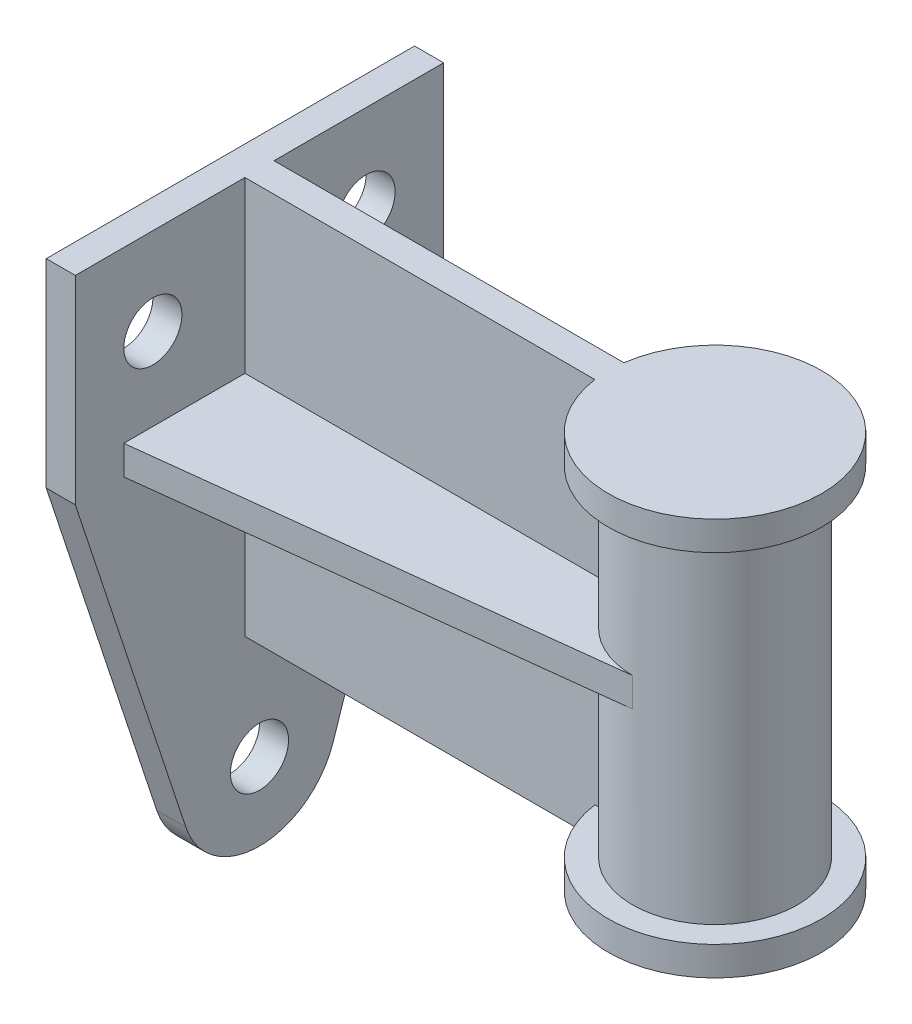
ISO-10303-21;
HEADER;
FILE_DESCRIPTION(('STEP AP214'),'2;1');
FILE_NAME('part.step','',(''),(''),'','','');
FILE_SCHEMA(('AUTOMOTIVE_DESIGN { 1 0 10303 214 1 1 1 1 }'));
ENDSEC;
DATA;
#1=APPLICATION_CONTEXT('core data for automotive mechanical design processes');
#2=APPLICATION_PROTOCOL_DEFINITION('international standard','automotive_design',2000,#1);
#3=PRODUCT_CONTEXT('',#1,'mechanical');
#4=PRODUCT('Part','Part','',(#3));
#5=PRODUCT_RELATED_PRODUCT_CATEGORY('part','',(#4));
#6=PRODUCT_DEFINITION_FORMATION('','',#4);
#7=PRODUCT_DEFINITION_CONTEXT('part definition',#1,'design');
#8=PRODUCT_DEFINITION('design','',#6,#7);
#9=PRODUCT_DEFINITION_SHAPE('','',#8);
#10=(LENGTH_UNIT() NAMED_UNIT(*) SI_UNIT(.MILLI.,.METRE.));
#11=(NAMED_UNIT(*) PLANE_ANGLE_UNIT() SI_UNIT($,.RADIAN.));
#12=(NAMED_UNIT(*) SI_UNIT($,.STERADIAN.) SOLID_ANGLE_UNIT());
#13=UNCERTAINTY_MEASURE_WITH_UNIT(LENGTH_MEASURE(1.E-05),#10,'distance_accuracy_value','');
#14=(GEOMETRIC_REPRESENTATION_CONTEXT(3) GLOBAL_UNCERTAINTY_ASSIGNED_CONTEXT((#13)) GLOBAL_UNIT_ASSIGNED_CONTEXT((#10,
#11,#12)) REPRESENTATION_CONTEXT('',''));
#15=CARTESIAN_POINT('',(0.,0.,0.));
#16=DIRECTION('',(0.,0.,1.));
#17=DIRECTION('',(1.,0.,0.));
#18=AXIS2_PLACEMENT_3D('',#15,#16,#17);
#19=CARTESIAN_POINT('',(0.,41.,0.));
#20=DIRECTION('',(0.,1.,0.));
#21=DIRECTION('',(0.,0.,1.));
#22=AXIS2_PLACEMENT_3D('',#19,#20,#21);
#23=PLANE('',#22);
#24=CARTESIAN_POINT('',(0.,41.,0.));
#25=DIRECTION('',(0.,1.,0.));
#26=DIRECTION('',(0.,0.,1.));
#27=AXIS2_PLACEMENT_3D('',#24,#25,#26);
#28=CIRCLE('',#27,17.);
#29=CARTESIAN_POINT('',(-7.7142620860374,41.,-15.148932651112));
#30=VERTEX_POINT('',#29);
#31=CARTESIAN_POINT('',(-16.7332005306815,41.,-3.));
#32=VERTEX_POINT('',#31);
#33=EDGE_CURVE('E61',#30,#32,#28,.T.);
#34=ORIENTED_EDGE('',*,*,#33,.T.);
#35=DIRECTION('',(1.,0.,0.));
#36=VECTOR('',#35,1.);
#37=CARTESIAN_POINT('',(0.,41.,-3.));
#38=LINE('',#37,#36);
#39=CARTESIAN_POINT('',(-94.,41.,-3.));
#40=VERTEX_POINT('',#39);
#41=EDGE_CURVE('E197',#40,#32,#38,.T.);
#42=ORIENTED_EDGE('',*,*,#41,.F.);
#43=DIRECTION('',(0.,0.,1.));
#44=VECTOR('',#43,1.);
#45=CARTESIAN_POINT('',(-94.,41.,0.));
#46=LINE('',#45,#44);
#47=CARTESIAN_POINT('',(-94.,41.,-28.));
#48=VERTEX_POINT('',#47);
#49=EDGE_CURVE('E11',#48,#40,#46,.T.);
#50=ORIENTED_EDGE('',*,*,#49,.F.);
#51=DIRECTION('',(0.989090177881817,0.,0.147311303088781));
#52=VECTOR('',#51,1.);
#53=CARTESIAN_POINT('',(2.03985828166519,41.,-13.696191319752));
#54=LINE('',#53,#52);
#55=EDGE_CURVE('E310',#48,#30,#54,.T.);
#56=ORIENTED_EDGE('',*,*,#55,.T.);
#57=EDGE_LOOP('',(#34,#42,#50,#56));
#58=FACE_BOUND('',#57,.T.);
#59=ADVANCED_FACE('F41',(#58),#23,.F.);
#60=CARTESIAN_POINT('',(-94.,41.,3.));
#61=VERTEX_POINT('',#60);
#62=CARTESIAN_POINT('',(-94.,41.,28.));
#63=VERTEX_POINT('',#62);
#64=EDGE_CURVE('E47',#61,#63,#46,.T.);
#65=ORIENTED_EDGE('',*,*,#64,.F.);
#66=DIRECTION('',(-1.,0.,0.));
#67=VECTOR('',#66,1.);
#68=CARTESIAN_POINT('',(0.,41.,3.));
#69=LINE('',#68,#67);
#70=CARTESIAN_POINT('',(-16.7332005306815,41.,3.));
#71=VERTEX_POINT('',#70);
#72=EDGE_CURVE('E186',#71,#61,#69,.T.);
#73=ORIENTED_EDGE('',*,*,#72,.F.);
#74=CARTESIAN_POINT('',(0.,41.,17.));
#75=VERTEX_POINT('',#74);
#76=EDGE_CURVE('E214',#71,#75,#28,.T.);
#77=ORIENTED_EDGE('',*,*,#76,.T.);
#78=DIRECTION('',(0.99322253932129,0.,-0.116228169495045));
#79=VECTOR('',#78,1.);
#80=CARTESIAN_POINT('',(1.96248743999107,41.,16.7703472144691));
#81=LINE('',#80,#79);
#82=EDGE_CURVE('E215',#63,#75,#81,.T.);
#83=ORIENTED_EDGE('',*,*,#82,.F.);
#84=EDGE_LOOP('',(#65,#73,#77,#83));
#85=FACE_BOUND('',#84,.T.);
#86=ADVANCED_FACE('F208',(#85),#23,.F.);
#87=CARTESIAN_POINT('',(0.,82.,0.));
#88=DIRECTION('',(0.,-1.,0.));
#89=DIRECTION('',(0.,0.,-1.));
#90=AXIS2_PLACEMENT_3D('',#87,#88,#89);
#91=CYLINDRICAL_SURFACE('',#90,17.);
#92=CARTESIAN_POINT('',(0.,6.,0.));
#93=DIRECTION('',(0.,1.,0.));
#94=DIRECTION('',(0.,0.,1.));
#95=AXIS2_PLACEMENT_3D('',#92,#93,#94);
#96=CIRCLE('',#95,17.);
#97=CARTESIAN_POINT('',(-16.7332005306815,6.,3.));
#98=VERTEX_POINT('',#97);
#99=CARTESIAN_POINT('',(-16.7332005306815,6.,-3.));
#100=VERTEX_POINT('',#99);
#101=EDGE_CURVE('E221',#98,#100,#96,.T.);
#102=ORIENTED_EDGE('',*,*,#101,.T.);
#103=DIRECTION('',(0.,-1.,0.));
#104=VECTOR('',#103,1.);
#105=CARTESIAN_POINT('',(-16.7332005306815,82.,-3.));
#106=LINE('',#105,#104);
#107=EDGE_CURVE('E354',#100,#32,#106,.F.);
#108=ORIENTED_EDGE('',*,*,#107,.T.);
#109=ORIENTED_EDGE('',*,*,#33,.F.);
#110=DIRECTION('',(0.,1.,0.));
#111=VECTOR('',#110,1.);
#112=CARTESIAN_POINT('',(-7.71426208603739,41.,-15.148932651112));
#113=LINE('',#112,#111);
#114=CARTESIAN_POINT('',(-7.71426208603739,47.,-15.148932651112));
#115=VERTEX_POINT('',#114);
#116=EDGE_CURVE('E304',#30,#115,#113,.T.);
#117=ORIENTED_EDGE('',*,*,#116,.T.);
#118=CARTESIAN_POINT('',(0.,47.,0.));
#119=DIRECTION('',(0.,1.,0.));
#120=DIRECTION('',(0.,0.,1.));
#121=AXIS2_PLACEMENT_3D('',#118,#119,#120);
#122=CIRCLE('',#121,17.);
#123=CARTESIAN_POINT('',(-16.7332005306815,47.,-3.));
#124=VERTEX_POINT('',#123);
#125=EDGE_CURVE('E319',#115,#124,#122,.T.);
#126=ORIENTED_EDGE('',*,*,#125,.T.);
#127=DIRECTION('',(0.,-1.,0.));
#128=VECTOR('',#127,1.);
#129=CARTESIAN_POINT('',(-16.7332005306815,82.,-3.));
#130=LINE('',#129,#128);
#131=CARTESIAN_POINT('',(-16.7332005306815,76.,-3.));
#132=VERTEX_POINT('',#131);
#133=EDGE_CURVE('E231',#124,#132,#130,.F.);
#134=ORIENTED_EDGE('',*,*,#133,.T.);
#135=CARTESIAN_POINT('',(0.,76.,0.));
#136=DIRECTION('',(0.,1.,0.));
#137=DIRECTION('',(0.,0.,1.));
#138=AXIS2_PLACEMENT_3D('',#135,#136,#137);
#139=CIRCLE('',#138,17.);
#140=CARTESIAN_POINT('',(-16.7332005306815,76.,3.));
#141=VERTEX_POINT('',#140);
#142=EDGE_CURVE('E217',#141,#132,#139,.T.);
#143=ORIENTED_EDGE('',*,*,#142,.F.);
#144=DIRECTION('',(0.,-1.,0.));
#145=VECTOR('',#144,1.);
#146=CARTESIAN_POINT('',(-16.7332005306815,82.,3.));
#147=LINE('',#146,#145);
#148=CARTESIAN_POINT('',(-16.7332005306815,47.,3.));
#149=VERTEX_POINT('',#148);
#150=EDGE_CURVE('E245',#149,#141,#147,.F.);
#151=ORIENTED_EDGE('',*,*,#150,.F.);
#152=CARTESIAN_POINT('',(0.,47.,0.));
#153=DIRECTION('',(0.,1.,0.));
#154=DIRECTION('',(0.,0.,1.));
#155=AXIS2_PLACEMENT_3D('',#152,#153,#154);
#156=CIRCLE('',#155,17.);
#157=CARTESIAN_POINT('',(0.,47.,17.));
#158=VERTEX_POINT('',#157);
#159=EDGE_CURVE('E297',#149,#158,#156,.T.);
#160=ORIENTED_EDGE('',*,*,#159,.T.);
#161=DIRECTION('',(0.,1.,0.));
#162=VECTOR('',#161,1.);
#163=CARTESIAN_POINT('',(0.,41.,17.));
#164=LINE('',#163,#162);
#165=EDGE_CURVE('E281',#75,#158,#164,.T.);
#166=ORIENTED_EDGE('',*,*,#165,.F.);
#167=ORIENTED_EDGE('',*,*,#76,.F.);
#168=DIRECTION('',(0.,-1.,0.));
#169=VECTOR('',#168,1.);
#170=CARTESIAN_POINT('',(-16.7332005306815,82.,3.));
#171=LINE('',#170,#169);
#172=EDGE_CURVE('E195',#71,#98,#171,.T.);
#173=ORIENTED_EDGE('',*,*,#172,.T.);
#174=EDGE_LOOP('',(#102,#108,#109,#117,#126,#134,#143,#151,#160,#166,#167,#173));
#175=FACE_BOUND('',#174,.T.);
#176=ADVANCED_FACE('F43',(#175),#91,.T.);
#177=CARTESIAN_POINT('',(0.,6.,0.));
#178=DIRECTION('',(0.,-1.,0.));
#179=DIRECTION('',(0.,0.,-1.));
#180=AXIS2_PLACEMENT_3D('',#177,#178,#179);
#181=CYLINDRICAL_SURFACE('',#180,22.);
#182=CARTESIAN_POINT('',(0.,0.,0.));
#183=DIRECTION('',(0.,1.,0.));
#184=DIRECTION('',(0.,0.,1.));
#185=AXIS2_PLACEMENT_3D('',#182,#183,#184);
#186=CIRCLE('',#185,22.);
#187=CARTESIAN_POINT('',(-21.7944947177034,0.,3.));
#188=VERTEX_POINT('',#187);
#189=CARTESIAN_POINT('',(-21.7944947177034,0.,-3.));
#190=VERTEX_POINT('',#189);
#191=EDGE_CURVE('E222',#188,#190,#186,.T.);
#192=ORIENTED_EDGE('',*,*,#191,.T.);
#193=DIRECTION('',(0.,-1.,0.));
#194=VECTOR('',#193,1.);
#195=CARTESIAN_POINT('',(-21.7944947177034,6.,-3.));
#196=LINE('',#195,#194);
#197=CARTESIAN_POINT('',(-21.7944947177034,6.,-3.));
#198=VERTEX_POINT('',#197);
#199=EDGE_CURVE('E365',#190,#198,#196,.F.);
#200=ORIENTED_EDGE('',*,*,#199,.T.);
#201=CARTESIAN_POINT('',(0.,6.,0.));
#202=DIRECTION('',(0.,1.,0.));
#203=DIRECTION('',(0.,0.,1.));
#204=AXIS2_PLACEMENT_3D('',#201,#202,#203);
#205=CIRCLE('',#204,22.);
#206=CARTESIAN_POINT('',(-21.7944947177034,6.,3.));
#207=VERTEX_POINT('',#206);
#208=EDGE_CURVE('E216',#207,#198,#205,.T.);
#209=ORIENTED_EDGE('',*,*,#208,.F.);
#210=DIRECTION('',(0.,-1.,0.));
#211=VECTOR('',#210,1.);
#212=CARTESIAN_POINT('',(-21.7944947177034,6.,3.));
#213=LINE('',#212,#211);
#214=EDGE_CURVE('E368',#207,#188,#213,.T.);
#215=ORIENTED_EDGE('',*,*,#214,.T.);
#216=EDGE_LOOP('',(#192,#200,#209,#215));
#217=FACE_BOUND('',#216,.T.);
#218=ADVANCED_FACE('F386',(#217),#181,.T.);
#219=CARTESIAN_POINT('',(0.,6.,0.));
#220=DIRECTION('',(0.,1.,0.));
#221=DIRECTION('',(0.,0.,1.));
#222=AXIS2_PLACEMENT_3D('',#219,#220,#221);
#223=PLANE('',#222);
#224=DIRECTION('',(-1.,0.,0.));
#225=VECTOR('',#224,1.);
#226=CARTESIAN_POINT('',(0.,6.,-3.));
#227=LINE('',#226,#225);
#228=EDGE_CURVE('E362',#100,#198,#227,.T.);
#229=ORIENTED_EDGE('',*,*,#228,.F.);
#230=ORIENTED_EDGE('',*,*,#101,.F.);
#231=DIRECTION('',(1.,0.,0.));
#232=VECTOR('',#231,1.);
#233=CARTESIAN_POINT('',(0.,6.,3.));
#234=LINE('',#233,#232);
#235=EDGE_CURVE('E371',#207,#98,#234,.T.);
#236=ORIENTED_EDGE('',*,*,#235,.F.);
#237=ORIENTED_EDGE('',*,*,#208,.T.);
#238=EDGE_LOOP('',(#229,#230,#236,#237));
#239=FACE_BOUND('',#238,.T.);
#240=ADVANCED_FACE('F387',(#239),#223,.T.);
#241=CARTESIAN_POINT('',(0.,0.,0.));
#242=DIRECTION('',(0.,1.,0.));
#243=DIRECTION('',(0.,0.,1.));
#244=AXIS2_PLACEMENT_3D('',#241,#242,#243);
#245=PLANE('',#244);
#246=ORIENTED_EDGE('',*,*,#191,.F.);
#247=DIRECTION('',(-1.,0.,0.));
#248=VECTOR('',#247,1.);
#249=CARTESIAN_POINT('',(0.,0.,3.));
#250=LINE('',#249,#248);
#251=CARTESIAN_POINT('',(-94.,0.,3.));
#252=VERTEX_POINT('',#251);
#253=EDGE_CURVE('E380',#188,#252,#250,.T.);
#254=ORIENTED_EDGE('',*,*,#253,.T.);
#255=DIRECTION('',(0.,0.,-1.));
#256=VECTOR('',#255,1.);
#257=CARTESIAN_POINT('',(-94.,0.,3.));
#258=LINE('',#257,#256);
#259=CARTESIAN_POINT('',(-94.,0.,-3.));
#260=VERTEX_POINT('',#259);
#261=EDGE_CURVE('E207',#252,#260,#258,.T.);
#262=ORIENTED_EDGE('',*,*,#261,.T.);
#263=DIRECTION('',(1.,0.,0.));
#264=VECTOR('',#263,1.);
#265=CARTESIAN_POINT('',(0.,0.,-3.));
#266=LINE('',#265,#264);
#267=EDGE_CURVE('E200',#260,#190,#266,.T.);
#268=ORIENTED_EDGE('',*,*,#267,.T.);
#269=EDGE_LOOP('',(#246,#254,#262,#268));
#270=FACE_BOUND('',#269,.T.);
#271=ADVANCED_FACE('F395',(#270),#245,.F.);
#272=CARTESIAN_POINT('',(0.,76.,0.));
#273=DIRECTION('',(0.,1.,0.));
#274=DIRECTION('',(0.,0.,1.));
#275=AXIS2_PLACEMENT_3D('',#272,#273,#274);
#276=CYLINDRICAL_SURFACE('',#275,22.);
#277=DIRECTION('',(0.,1.,0.));
#278=VECTOR('',#277,1.);
#279=CARTESIAN_POINT('',(-21.7944947177034,76.,-3.));
#280=LINE('',#279,#278);
#281=CARTESIAN_POINT('',(-21.7944947177034,82.,-3.));
#282=VERTEX_POINT('',#281);
#283=CARTESIAN_POINT('',(-21.7944947177034,76.,-3.));
#284=VERTEX_POINT('',#283);
#285=EDGE_CURVE('E240',#282,#284,#280,.F.);
#286=ORIENTED_EDGE('',*,*,#285,.F.);
#287=CARTESIAN_POINT('',(0.,82.,0.));
#288=DIRECTION('',(0.,1.,0.));
#289=DIRECTION('',(0.,0.,1.));
#290=AXIS2_PLACEMENT_3D('',#287,#288,#289);
#291=CIRCLE('',#290,22.);
#292=CARTESIAN_POINT('',(-21.7944947177034,82.,3.));
#293=VERTEX_POINT('',#292);
#294=EDGE_CURVE('E229',#293,#282,#291,.T.);
#295=ORIENTED_EDGE('',*,*,#294,.F.);
#296=DIRECTION('',(0.,1.,0.));
#297=VECTOR('',#296,1.);
#298=CARTESIAN_POINT('',(-21.7944947177034,76.,3.));
#299=LINE('',#298,#297);
#300=CARTESIAN_POINT('',(-21.7944947177034,76.,3.));
#301=VERTEX_POINT('',#300);
#302=EDGE_CURVE('E242',#293,#301,#299,.F.);
#303=ORIENTED_EDGE('',*,*,#302,.T.);
#304=CARTESIAN_POINT('',(0.,76.,0.));
#305=DIRECTION('',(0.,1.,0.));
#306=DIRECTION('',(0.,0.,1.));
#307=AXIS2_PLACEMENT_3D('',#304,#305,#306);
#308=CIRCLE('',#307,22.);
#309=EDGE_CURVE('E223',#301,#284,#308,.T.);
#310=ORIENTED_EDGE('',*,*,#309,.T.);
#311=EDGE_LOOP('',(#286,#295,#303,#310));
#312=FACE_BOUND('',#311,.T.);
#313=ADVANCED_FACE('F420',(#312),#276,.T.);
#314=CARTESIAN_POINT('',(0.,76.,0.));
#315=DIRECTION('',(0.,1.,0.));
#316=DIRECTION('',(0.,0.,1.));
#317=AXIS2_PLACEMENT_3D('',#314,#315,#316);
#318=PLANE('',#317);
#319=ORIENTED_EDGE('',*,*,#142,.T.);
#320=DIRECTION('',(-1.,0.,0.));
#321=VECTOR('',#320,1.);
#322=CARTESIAN_POINT('',(0.,76.,-3.));
#323=LINE('',#322,#321);
#324=EDGE_CURVE('E239',#132,#284,#323,.T.);
#325=ORIENTED_EDGE('',*,*,#324,.T.);
#326=ORIENTED_EDGE('',*,*,#309,.F.);
#327=DIRECTION('',(-1.,0.,0.));
#328=VECTOR('',#327,1.);
#329=CARTESIAN_POINT('',(0.,76.,3.));
#330=LINE('',#329,#328);
#331=EDGE_CURVE('E250',#141,#301,#330,.T.);
#332=ORIENTED_EDGE('',*,*,#331,.F.);
#333=EDGE_LOOP('',(#319,#325,#326,#332));
#334=FACE_BOUND('',#333,.T.);
#335=ADVANCED_FACE('F424',(#334),#318,.F.);
#336=CARTESIAN_POINT('',(0.,82.,0.));
#337=DIRECTION('',(0.,1.,0.));
#338=DIRECTION('',(0.,0.,1.));
#339=AXIS2_PLACEMENT_3D('',#336,#337,#338);
#340=PLANE('',#339);
#341=ORIENTED_EDGE('',*,*,#294,.T.);
#342=DIRECTION('',(-1.,0.,0.));
#343=VECTOR('',#342,1.);
#344=CARTESIAN_POINT('',(0.,82.,-3.));
#345=LINE('',#344,#343);
#346=CARTESIAN_POINT('',(-94.,82.,-3.));
#347=VERTEX_POINT('',#346);
#348=EDGE_CURVE('E285',#282,#347,#345,.T.);
#349=ORIENTED_EDGE('',*,*,#348,.T.);
#350=DIRECTION('',(0.,0.,-1.));
#351=VECTOR('',#350,1.);
#352=CARTESIAN_POINT('',(-94.,82.,0.));
#353=LINE('',#352,#351);
#354=CARTESIAN_POINT('',(-94.,82.,-38.));
#355=VERTEX_POINT('',#354);
#356=EDGE_CURVE('E276',#347,#355,#353,.T.);
#357=ORIENTED_EDGE('',*,*,#356,.T.);
#358=DIRECTION('',(1.,0.,0.));
#359=VECTOR('',#358,1.);
#360=CARTESIAN_POINT('',(0.,82.,-38.));
#361=LINE('',#360,#359);
#362=CARTESIAN_POINT('',(-100.,82.,-38.));
#363=VERTEX_POINT('',#362);
#364=EDGE_CURVE('E277',#363,#355,#361,.T.);
#365=ORIENTED_EDGE('',*,*,#364,.F.);
#366=DIRECTION('',(0.,0.,-1.));
#367=VECTOR('',#366,1.);
#368=CARTESIAN_POINT('',(-100.,82.,0.));
#369=LINE('',#368,#367);
#370=CARTESIAN_POINT('',(-100.,82.,38.));
#371=VERTEX_POINT('',#370);
#372=EDGE_CURVE('E274',#371,#363,#369,.T.);
#373=ORIENTED_EDGE('',*,*,#372,.F.);
#374=DIRECTION('',(1.,0.,0.));
#375=VECTOR('',#374,1.);
#376=CARTESIAN_POINT('',(0.,82.,38.));
#377=LINE('',#376,#375);
#378=CARTESIAN_POINT('',(-94.,82.,38.));
#379=VERTEX_POINT('',#378);
#380=EDGE_CURVE('E272',#371,#379,#377,.T.);
#381=ORIENTED_EDGE('',*,*,#380,.T.);
#382=DIRECTION('',(0.,0.,-1.));
#383=VECTOR('',#382,1.);
#384=CARTESIAN_POINT('',(-94.,82.,0.));
#385=LINE('',#384,#383);
#386=CARTESIAN_POINT('',(-94.,82.,3.));
#387=VERTEX_POINT('',#386);
#388=EDGE_CURVE('E269',#379,#387,#385,.T.);
#389=ORIENTED_EDGE('',*,*,#388,.T.);
#390=DIRECTION('',(-1.,0.,0.));
#391=VECTOR('',#390,1.);
#392=CARTESIAN_POINT('',(0.,82.,3.));
#393=LINE('',#392,#391);
#394=EDGE_CURVE('E264',#293,#387,#393,.T.);
#395=ORIENTED_EDGE('',*,*,#394,.F.);
#396=EDGE_LOOP('',(#341,#349,#357,#365,#373,#381,#389,#395));
#397=FACE_BOUND('',#396,.T.);
#398=ADVANCED_FACE('F415',(#397),#340,.T.);
#399=CARTESIAN_POINT('',(0.,41.,-3.));
#400=DIRECTION('',(0.,0.,-1.));
#401=DIRECTION('',(-1.,0.,0.));
#402=AXIS2_PLACEMENT_3D('',#399,#400,#401);
#403=PLANE('',#402);
#404=DIRECTION('',(1.,0.,0.));
#405=VECTOR('',#404,1.);
#406=CARTESIAN_POINT('',(0.,47.,-3.));
#407=LINE('',#406,#405);
#408=CARTESIAN_POINT('',(-94.,47.,-3.));
#409=VERTEX_POINT('',#408);
#410=EDGE_CURVE('E309',#409,#124,#407,.T.);
#411=ORIENTED_EDGE('',*,*,#410,.F.);
#412=DIRECTION('',(0.,1.,0.));
#413=VECTOR('',#412,1.);
#414=CARTESIAN_POINT('',(-94.,41.,-3.));
#415=LINE('',#414,#413);
#416=EDGE_CURVE('E252',#409,#347,#415,.T.);
#417=ORIENTED_EDGE('',*,*,#416,.T.);
#418=ORIENTED_EDGE('',*,*,#348,.F.);
#419=ORIENTED_EDGE('',*,*,#285,.T.);
#420=ORIENTED_EDGE('',*,*,#324,.F.);
#421=ORIENTED_EDGE('',*,*,#133,.F.);
#422=EDGE_LOOP('',(#411,#417,#418,#419,#420,#421));
#423=FACE_BOUND('',#422,.T.);
#424=ADVANCED_FACE('F403',(#423),#403,.T.);
#425=CARTESIAN_POINT('',(0.,41.,3.));
#426=DIRECTION('',(0.,0.,-1.));
#427=DIRECTION('',(-1.,0.,0.));
#428=AXIS2_PLACEMENT_3D('',#425,#426,#427);
#429=PLANE('',#428);
#430=DIRECTION('',(0.,1.,0.));
#431=VECTOR('',#430,1.);
#432=CARTESIAN_POINT('',(-94.,41.,3.));
#433=LINE('',#432,#431);
#434=CARTESIAN_POINT('',(-94.,47.,3.));
#435=VERTEX_POINT('',#434);
#436=EDGE_CURVE('E249',#435,#387,#433,.T.);
#437=ORIENTED_EDGE('',*,*,#436,.F.);
#438=DIRECTION('',(-1.,0.,0.));
#439=VECTOR('',#438,1.);
#440=CARTESIAN_POINT('',(0.,47.,3.));
#441=LINE('',#440,#439);
#442=EDGE_CURVE('E296',#149,#435,#441,.T.);
#443=ORIENTED_EDGE('',*,*,#442,.F.);
#444=ORIENTED_EDGE('',*,*,#150,.T.);
#445=ORIENTED_EDGE('',*,*,#331,.T.);
#446=ORIENTED_EDGE('',*,*,#302,.F.);
#447=ORIENTED_EDGE('',*,*,#394,.T.);
#448=EDGE_LOOP('',(#437,#443,#444,#445,#446,#447));
#449=FACE_BOUND('',#448,.T.);
#450=ADVANCED_FACE('F418',(#449),#429,.F.);
#451=CARTESIAN_POINT('',(-94.,41.,0.));
#452=DIRECTION('',(1.,0.,0.));
#453=DIRECTION('',(0.,0.,-1.));
#454=AXIS2_PLACEMENT_3D('',#451,#452,#453);
#455=PLANE('',#454);
#456=DIRECTION('',(0.,-1.,0.));
#457=VECTOR('',#456,1.);
#458=CARTESIAN_POINT('',(-94.,41.,-3.));
#459=LINE('',#458,#457);
#460=EDGE_CURVE('E210',#40,#260,#459,.T.);
#461=ORIENTED_EDGE('',*,*,#460,.T.);
#462=ORIENTED_EDGE('',*,*,#261,.F.);
#463=DIRECTION('',(0.,-1.,0.));
#464=VECTOR('',#463,1.);
#465=CARTESIAN_POINT('',(-94.,41.,3.));
#466=LINE('',#465,#464);
#467=EDGE_CURVE('E57',#61,#252,#466,.T.);
#468=ORIENTED_EDGE('',*,*,#467,.F.);
#469=ORIENTED_EDGE('',*,*,#64,.T.);
#470=DIRECTION('',(0.,1.,0.));
#471=VECTOR('',#470,1.);
#472=CARTESIAN_POINT('',(-94.,41.,28.));
#473=LINE('',#472,#471);
#474=CARTESIAN_POINT('',(-94.,47.,28.));
#475=VERTEX_POINT('',#474);
#476=EDGE_CURVE('E288',#63,#475,#473,.T.);
#477=ORIENTED_EDGE('',*,*,#476,.T.);
#478=DIRECTION('',(0.,0.,1.));
#479=VECTOR('',#478,1.);
#480=CARTESIAN_POINT('',(-94.,47.,0.));
#481=LINE('',#480,#479);
#482=EDGE_CURVE('E298',#435,#475,#481,.T.);
#483=ORIENTED_EDGE('',*,*,#482,.F.);
#484=ORIENTED_EDGE('',*,*,#436,.T.);
#485=ORIENTED_EDGE('',*,*,#388,.F.);
#486=DIRECTION('',(0.,1.,0.));
#487=VECTOR('',#486,1.);
#488=CARTESIAN_POINT('',(-94.,41.,38.));
#489=LINE('',#488,#487);
#490=CARTESIAN_POINT('',(-94.,41.,38.));
#491=VERTEX_POINT('',#490);
#492=EDGE_CURVE('E262',#491,#379,#489,.T.);
#493=ORIENTED_EDGE('',*,*,#492,.F.);
#494=DIRECTION('',(0.,-0.949500388523264,-0.313765855685688));
#495=VECTOR('',#494,1.);
#496=CARTESIAN_POINT('',(-94.,-7.28458097143695,22.0441846595868));
#497=LINE('',#496,#495);
#498=CARTESIAN_POINT('',(-94.,-28.020253690971,15.1920062163722));
#499=VERTEX_POINT('',#498);
#500=EDGE_CURVE('E321',#491,#499,#497,.T.);
#501=ORIENTED_EDGE('',*,*,#500,.T.);
#502=CARTESIAN_POINT('',(-94.,-23.,0.));
#503=DIRECTION('',(-1.,0.,0.));
#504=DIRECTION('',(0.,0.,1.));
#505=AXIS2_PLACEMENT_3D('',#502,#503,#504);
#506=CIRCLE('',#505,16.);
#507=CARTESIAN_POINT('',(-94.,-28.020253690971,-15.1920062163722));
#508=VERTEX_POINT('',#507);
#509=EDGE_CURVE('E342',#508,#499,#506,.T.);
#510=ORIENTED_EDGE('',*,*,#509,.F.);
#511=DIRECTION('',(0.,-0.949500388523264,0.313765855685688));
#512=VECTOR('',#511,1.);
#513=CARTESIAN_POINT('',(-94.,-7.28458097143695,-22.0441846595868));
#514=LINE('',#513,#512);
#515=CARTESIAN_POINT('',(-94.,41.,-38.));
#516=VERTEX_POINT('',#515);
#517=EDGE_CURVE('E341',#516,#508,#514,.T.);
#518=ORIENTED_EDGE('',*,*,#517,.F.);
#519=DIRECTION('',(0.,1.,0.));
#520=VECTOR('',#519,1.);
#521=CARTESIAN_POINT('',(-94.,41.,-38.));
#522=LINE('',#521,#520);
#523=EDGE_CURVE('E254',#516,#355,#522,.T.);
#524=ORIENTED_EDGE('',*,*,#523,.T.);
#525=ORIENTED_EDGE('',*,*,#356,.F.);
#526=ORIENTED_EDGE('',*,*,#416,.F.);
#527=DIRECTION('',(0.,0.,-1.));
#528=VECTOR('',#527,1.);
#529=CARTESIAN_POINT('',(-94.,47.,0.));
#530=LINE('',#529,#528);
#531=CARTESIAN_POINT('',(-94.,47.,-28.));
#532=VERTEX_POINT('',#531);
#533=EDGE_CURVE('E312',#409,#532,#530,.T.);
#534=ORIENTED_EDGE('',*,*,#533,.T.);
#535=DIRECTION('',(0.,1.,0.));
#536=VECTOR('',#535,1.);
#537=CARTESIAN_POINT('',(-94.,41.,-28.));
#538=LINE('',#537,#536);
#539=EDGE_CURVE('E303',#48,#532,#538,.T.);
#540=ORIENTED_EDGE('',*,*,#539,.F.);
#541=ORIENTED_EDGE('',*,*,#49,.T.);
#542=EDGE_LOOP('',(#461,#462,#468,#469,#477,#483,#484,#485,#493,#501,#510,#518,#524,#525,#526,
#534,#540,#541));
#543=FACE_BOUND('',#542,.T.);
#544=CARTESIAN_POINT('',(-94.,64.,-22.));
#545=DIRECTION('',(-1.,0.,0.));
#546=DIRECTION('',(0.,0.,1.));
#547=AXIS2_PLACEMENT_3D('',#544,#545,#546);
#548=CIRCLE('',#547,6.);
#549=CARTESIAN_POINT('',(-94.,64.,-16.));
#550=VERTEX_POINT('',#549);
#551=EDGE_CURVE('E339',#550,#550,#548,.T.);
#552=ORIENTED_EDGE('',*,*,#551,.T.);
#553=EDGE_LOOP('',(#552));
#554=FACE_BOUND('',#553,.T.);
#555=CARTESIAN_POINT('',(-94.,64.,22.));
#556=DIRECTION('',(-1.,0.,0.));
#557=DIRECTION('',(0.,0.,1.));
#558=AXIS2_PLACEMENT_3D('',#555,#556,#557);
#559=CIRCLE('',#558,6.);
#560=CARTESIAN_POINT('',(-94.,64.,28.));
#561=VERTEX_POINT('',#560);
#562=EDGE_CURVE('E355',#561,#561,#559,.T.);
#563=ORIENTED_EDGE('',*,*,#562,.T.);
#564=EDGE_LOOP('',(#563));
#565=FACE_BOUND('',#564,.T.);
#566=CARTESIAN_POINT('',(-94.,-23.,0.));
#567=DIRECTION('',(-1.,0.,0.));
#568=DIRECTION('',(0.,0.,1.));
#569=AXIS2_PLACEMENT_3D('',#566,#567,#568);
#570=CIRCLE('',#569,6.);
#571=CARTESIAN_POINT('',(-94.,-23.,6.00000000000002));
#572=VERTEX_POINT('',#571);
#573=EDGE_CURVE('E329',#572,#572,#570,.T.);
#574=ORIENTED_EDGE('',*,*,#573,.T.);
#575=EDGE_LOOP('',(#574));
#576=FACE_BOUND('',#575,.T.);
#577=ADVANCED_FACE('F205',(#543,#554,#565,#576),#455,.T.);
#578=CARTESIAN_POINT('',(0.,41.,38.));
#579=DIRECTION('',(0.,0.,1.));
#580=DIRECTION('',(1.,0.,0.));
#581=AXIS2_PLACEMENT_3D('',#578,#579,#580);
#582=PLANE('',#581);
#583=ORIENTED_EDGE('',*,*,#380,.F.);
#584=DIRECTION('',(0.,1.,0.));
#585=VECTOR('',#584,1.);
#586=CARTESIAN_POINT('',(-100.,41.,38.));
#587=LINE('',#586,#585);
#588=CARTESIAN_POINT('',(-100.,41.,38.));
#589=VERTEX_POINT('',#588);
#590=EDGE_CURVE('E256',#589,#371,#587,.T.);
#591=ORIENTED_EDGE('',*,*,#590,.F.);
#592=DIRECTION('',(1.,0.,0.));
#593=VECTOR('',#592,1.);
#594=CARTESIAN_POINT('',(0.,41.,38.));
#595=LINE('',#594,#593);
#596=EDGE_CURVE('E251',#589,#491,#595,.T.);
#597=ORIENTED_EDGE('',*,*,#596,.T.);
#598=ORIENTED_EDGE('',*,*,#492,.T.);
#599=EDGE_LOOP('',(#583,#591,#597,#598));
#600=FACE_BOUND('',#599,.T.);
#601=ADVANCED_FACE('F460',(#600),#582,.T.);
#602=CARTESIAN_POINT('',(-100.,41.,0.));
#603=DIRECTION('',(1.,0.,0.));
#604=DIRECTION('',(0.,0.,-1.));
#605=AXIS2_PLACEMENT_3D('',#602,#603,#604);
#606=PLANE('',#605);
#607=CARTESIAN_POINT('',(-100.,64.,-22.));
#608=DIRECTION('',(-1.,0.,0.));
#609=DIRECTION('',(0.,0.,1.));
#610=AXIS2_PLACEMENT_3D('',#607,#608,#609);
#611=CIRCLE('',#610,6.);
#612=CARTESIAN_POINT('',(-100.,64.,-16.));
#613=VERTEX_POINT('',#612);
#614=EDGE_CURVE('E358',#613,#613,#611,.T.);
#615=ORIENTED_EDGE('',*,*,#614,.F.);
#616=EDGE_LOOP('',(#615));
#617=FACE_BOUND('',#616,.T.);
#618=CARTESIAN_POINT('',(-100.,64.,22.));
#619=DIRECTION('',(-1.,0.,0.));
#620=DIRECTION('',(0.,0.,1.));
#621=AXIS2_PLACEMENT_3D('',#618,#619,#620);
#622=CIRCLE('',#621,6.);
#623=CARTESIAN_POINT('',(-100.,64.,28.));
#624=VERTEX_POINT('',#623);
#625=EDGE_CURVE('E349',#624,#624,#622,.T.);
#626=ORIENTED_EDGE('',*,*,#625,.F.);
#627=EDGE_LOOP('',(#626));
#628=FACE_BOUND('',#627,.T.);
#629=ORIENTED_EDGE('',*,*,#372,.T.);
#630=DIRECTION('',(0.,1.,0.));
#631=VECTOR('',#630,1.);
#632=CARTESIAN_POINT('',(-100.,41.,-38.));
#633=LINE('',#632,#631);
#634=CARTESIAN_POINT('',(-100.,41.,-38.));
#635=VERTEX_POINT('',#634);
#636=EDGE_CURVE('E257',#635,#363,#633,.T.);
#637=ORIENTED_EDGE('',*,*,#636,.F.);
#638=DIRECTION('',(0.,-0.949500388523264,0.313765855685688));
#639=VECTOR('',#638,1.);
#640=CARTESIAN_POINT('',(-100.,-7.28458097143695,-22.0441846595868));
#641=LINE('',#640,#639);
#642=CARTESIAN_POINT('',(-100.,-28.020253690971,-15.1920062163722));
#643=VERTEX_POINT('',#642);
#644=EDGE_CURVE('E334',#635,#643,#641,.T.);
#645=ORIENTED_EDGE('',*,*,#644,.T.);
#646=CARTESIAN_POINT('',(-100.,-23.,0.));
#647=DIRECTION('',(-1.,0.,0.));
#648=DIRECTION('',(0.,0.,1.));
#649=AXIS2_PLACEMENT_3D('',#646,#647,#648);
#650=CIRCLE('',#649,16.);
#651=CARTESIAN_POINT('',(-100.,-28.020253690971,15.1920062163722));
#652=VERTEX_POINT('',#651);
#653=EDGE_CURVE('E326',#643,#652,#650,.T.);
#654=ORIENTED_EDGE('',*,*,#653,.T.);
#655=DIRECTION('',(0.,-0.949500388523264,-0.313765855685688));
#656=VECTOR('',#655,1.);
#657=CARTESIAN_POINT('',(-100.,-7.28458097143695,22.0441846595868));
#658=LINE('',#657,#656);
#659=EDGE_CURVE('E327',#589,#652,#658,.T.);
#660=ORIENTED_EDGE('',*,*,#659,.F.);
#661=ORIENTED_EDGE('',*,*,#590,.T.);
#662=EDGE_LOOP('',(#629,#637,#645,#654,#660,#661));
#663=FACE_BOUND('',#662,.T.);
#664=CARTESIAN_POINT('',(-100.,-23.,0.));
#665=DIRECTION('',(-1.,0.,0.));
#666=DIRECTION('',(0.,0.,1.));
#667=AXIS2_PLACEMENT_3D('',#664,#665,#666);
#668=CIRCLE('',#667,6.);
#669=CARTESIAN_POINT('',(-100.,-23.,6.00000000000003));
#670=VERTEX_POINT('',#669);
#671=EDGE_CURVE('E337',#670,#670,#668,.T.);
#672=ORIENTED_EDGE('',*,*,#671,.F.);
#673=EDGE_LOOP('',(#672));
#674=FACE_BOUND('',#673,.T.);
#675=ADVANCED_FACE('F442',(#617,#628,#663,#674),#606,.F.);
#676=CARTESIAN_POINT('',(0.,41.,-38.));
#677=DIRECTION('',(0.,0.,1.));
#678=DIRECTION('',(1.,0.,0.));
#679=AXIS2_PLACEMENT_3D('',#676,#677,#678);
#680=PLANE('',#679);
#681=ORIENTED_EDGE('',*,*,#364,.T.);
#682=ORIENTED_EDGE('',*,*,#523,.F.);
#683=DIRECTION('',(1.,0.,0.));
#684=VECTOR('',#683,1.);
#685=CARTESIAN_POINT('',(0.,41.,-38.));
#686=LINE('',#685,#684);
#687=EDGE_CURVE('E270',#635,#516,#686,.T.);
#688=ORIENTED_EDGE('',*,*,#687,.F.);
#689=ORIENTED_EDGE('',*,*,#636,.T.);
#690=EDGE_LOOP('',(#681,#682,#688,#689));
#691=FACE_BOUND('',#690,.T.);
#692=ADVANCED_FACE('F434',(#691),#680,.F.);
#693=CARTESIAN_POINT('',(1.96248743999107,41.,16.7703472144691));
#694=DIRECTION('',(0.116228169495045,0.,0.99322253932129));
#695=DIRECTION('',(0.99322253932129,0.,-0.116228169495045));
#696=AXIS2_PLACEMENT_3D('',#693,#694,#695);
#697=PLANE('',#696);
#698=DIRECTION('',(0.99322253932129,0.,-0.116228169495045));
#699=VECTOR('',#698,1.);
#700=CARTESIAN_POINT('',(1.96248743999107,47.,16.7703472144691));
#701=LINE('',#700,#699);
#702=EDGE_CURVE('E291',#475,#158,#701,.T.);
#703=ORIENTED_EDGE('',*,*,#702,.F.);
#704=ORIENTED_EDGE('',*,*,#476,.F.);
#705=ORIENTED_EDGE('',*,*,#82,.T.);
#706=ORIENTED_EDGE('',*,*,#165,.T.);
#707=EDGE_LOOP('',(#703,#704,#705,#706));
#708=FACE_BOUND('',#707,.T.);
#709=ADVANCED_FACE('F433',(#708),#697,.T.);
#710=CARTESIAN_POINT('',(0.,47.,0.));
#711=DIRECTION('',(0.,1.,0.));
#712=DIRECTION('',(0.,0.,1.));
#713=AXIS2_PLACEMENT_3D('',#710,#711,#712);
#714=PLANE('',#713);
#715=ORIENTED_EDGE('',*,*,#159,.F.);
#716=ORIENTED_EDGE('',*,*,#442,.T.);
#717=ORIENTED_EDGE('',*,*,#482,.T.);
#718=ORIENTED_EDGE('',*,*,#702,.T.);
#719=EDGE_LOOP('',(#715,#716,#717,#718));
#720=FACE_BOUND('',#719,.T.);
#721=ADVANCED_FACE('F426',(#720),#714,.T.);
#722=CARTESIAN_POINT('',(2.03985828166519,41.,-13.696191319752));
#723=DIRECTION('',(-0.147311303088781,0.,0.989090177881817));
#724=DIRECTION('',(0.989090177881818,0.,0.147311303088781));
#725=AXIS2_PLACEMENT_3D('',#722,#723,#724);
#726=PLANE('',#725);
#727=DIRECTION('',(0.989090177881817,0.,0.147311303088781));
#728=VECTOR('',#727,1.);
#729=CARTESIAN_POINT('',(2.03985828166519,47.,-13.696191319752));
#730=LINE('',#729,#728);
#731=EDGE_CURVE('E314',#532,#115,#730,.T.);
#732=ORIENTED_EDGE('',*,*,#731,.T.);
#733=ORIENTED_EDGE('',*,*,#116,.F.);
#734=ORIENTED_EDGE('',*,*,#55,.F.);
#735=ORIENTED_EDGE('',*,*,#539,.T.);
#736=EDGE_LOOP('',(#732,#733,#734,#735));
#737=FACE_BOUND('',#736,.T.);
#738=ADVANCED_FACE('F400',(#737),#726,.F.);
#739=CARTESIAN_POINT('',(0.,47.,0.));
#740=DIRECTION('',(0.,1.,0.));
#741=DIRECTION('',(0.,0.,1.));
#742=AXIS2_PLACEMENT_3D('',#739,#740,#741);
#743=PLANE('',#742);
#744=ORIENTED_EDGE('',*,*,#125,.F.);
#745=ORIENTED_EDGE('',*,*,#731,.F.);
#746=ORIENTED_EDGE('',*,*,#533,.F.);
#747=ORIENTED_EDGE('',*,*,#410,.T.);
#748=EDGE_LOOP('',(#744,#745,#746,#747));
#749=FACE_BOUND('',#748,.T.);
#750=ADVANCED_FACE('F409',(#749),#743,.T.);
#751=CARTESIAN_POINT('',(-94.,-7.28458097143695,-22.0441846595868));
#752=DIRECTION('',(0.,-0.313765855685687,-0.949500388523263));
#753=DIRECTION('',(0.,0.949500388523264,-0.313765855685688));
#754=AXIS2_PLACEMENT_3D('',#751,#752,#753);
#755=PLANE('',#754);
#756=ORIENTED_EDGE('',*,*,#644,.F.);
#757=ORIENTED_EDGE('',*,*,#687,.T.);
#758=ORIENTED_EDGE('',*,*,#517,.T.);
#759=DIRECTION('',(-1.,0.,0.));
#760=VECTOR('',#759,1.);
#761=CARTESIAN_POINT('',(-94.,-28.020253690971,-15.1920062163722));
#762=LINE('',#761,#760);
#763=EDGE_CURVE('E325',#508,#643,#762,.T.);
#764=ORIENTED_EDGE('',*,*,#763,.T.);
#765=EDGE_LOOP('',(#756,#757,#758,#764));
#766=FACE_BOUND('',#765,.T.);
#767=ADVANCED_FACE('F551',(#766),#755,.T.);
#768=CARTESIAN_POINT('',(-94.,-7.28458097143695,22.0441846595868));
#769=DIRECTION('',(0.,0.313765855685688,-0.949500388523263));
#770=DIRECTION('',(0.,0.949500388523264,0.313765855685688));
#771=AXIS2_PLACEMENT_3D('',#768,#769,#770);
#772=PLANE('',#771);
#773=ORIENTED_EDGE('',*,*,#659,.T.);
#774=DIRECTION('',(-1.,0.,0.));
#775=VECTOR('',#774,1.);
#776=CARTESIAN_POINT('',(-94.,-28.020253690971,15.1920062163722));
#777=LINE('',#776,#775);
#778=EDGE_CURVE('E318',#499,#652,#777,.T.);
#779=ORIENTED_EDGE('',*,*,#778,.F.);
#780=ORIENTED_EDGE('',*,*,#500,.F.);
#781=ORIENTED_EDGE('',*,*,#596,.F.);
#782=EDGE_LOOP('',(#773,#779,#780,#781));
#783=FACE_BOUND('',#782,.T.);
#784=ADVANCED_FACE('F543',(#783),#772,.F.);
#785=CARTESIAN_POINT('',(-94.,-23.,0.));
#786=DIRECTION('',(-1.,0.,0.));
#787=DIRECTION('',(0.,0.,1.));
#788=AXIS2_PLACEMENT_3D('',#785,#786,#787);
#789=CYLINDRICAL_SURFACE('',#788,6.);
#790=ORIENTED_EDGE('',*,*,#573,.F.);
#791=EDGE_LOOP('',(#790));
#792=FACE_BOUND('',#791,.T.);
#793=ORIENTED_EDGE('',*,*,#671,.T.);
#794=EDGE_LOOP('',(#793));
#795=FACE_BOUND('',#794,.T.);
#796=ADVANCED_FACE('F534',(#792,#795),#789,.F.);
#797=CARTESIAN_POINT('',(-94.,-23.,0.));
#798=DIRECTION('',(-1.,0.,0.));
#799=DIRECTION('',(0.,0.,1.));
#800=AXIS2_PLACEMENT_3D('',#797,#798,#799);
#801=CYLINDRICAL_SURFACE('',#800,16.);
#802=ORIENTED_EDGE('',*,*,#653,.F.);
#803=ORIENTED_EDGE('',*,*,#763,.F.);
#804=ORIENTED_EDGE('',*,*,#509,.T.);
#805=ORIENTED_EDGE('',*,*,#778,.T.);
#806=EDGE_LOOP('',(#802,#803,#804,#805));
#807=FACE_BOUND('',#806,.T.);
#808=ADVANCED_FACE('F521',(#807),#801,.T.);
#809=CARTESIAN_POINT('',(-94.,64.,22.));
#810=DIRECTION('',(-1.,0.,0.));
#811=DIRECTION('',(0.,0.,1.));
#812=AXIS2_PLACEMENT_3D('',#809,#810,#811);
#813=CYLINDRICAL_SURFACE('',#812,6.);
#814=ORIENTED_EDGE('',*,*,#562,.F.);
#815=EDGE_LOOP('',(#814));
#816=FACE_BOUND('',#815,.T.);
#817=ORIENTED_EDGE('',*,*,#625,.T.);
#818=EDGE_LOOP('',(#817));
#819=FACE_BOUND('',#818,.T.);
#820=ADVANCED_FACE('F517',(#816,#819),#813,.F.);
#821=CARTESIAN_POINT('',(-94.,64.,-22.));
#822=DIRECTION('',(-1.,0.,0.));
#823=DIRECTION('',(0.,0.,1.));
#824=AXIS2_PLACEMENT_3D('',#821,#822,#823);
#825=CYLINDRICAL_SURFACE('',#824,6.);
#826=ORIENTED_EDGE('',*,*,#551,.F.);
#827=EDGE_LOOP('',(#826));
#828=FACE_BOUND('',#827,.T.);
#829=ORIENTED_EDGE('',*,*,#614,.T.);
#830=EDGE_LOOP('',(#829));
#831=FACE_BOUND('',#830,.T.);
#832=ADVANCED_FACE('F491',(#828,#831),#825,.F.);
#833=CARTESIAN_POINT('',(0.,41.,-3.));
#834=DIRECTION('',(0.,0.,-1.));
#835=DIRECTION('',(-1.,0.,0.));
#836=AXIS2_PLACEMENT_3D('',#833,#834,#835);
#837=PLANE('',#836);
#838=ORIENTED_EDGE('',*,*,#107,.F.);
#839=ORIENTED_EDGE('',*,*,#228,.T.);
#840=ORIENTED_EDGE('',*,*,#199,.F.);
#841=ORIENTED_EDGE('',*,*,#267,.F.);
#842=ORIENTED_EDGE('',*,*,#460,.F.);
#843=ORIENTED_EDGE('',*,*,#41,.T.);
#844=EDGE_LOOP('',(#838,#839,#840,#841,#842,#843));
#845=FACE_BOUND('',#844,.T.);
#846=ADVANCED_FACE('F379',(#845),#837,.T.);
#847=CARTESIAN_POINT('',(0.,41.,3.));
#848=DIRECTION('',(0.,0.,1.));
#849=DIRECTION('',(1.,0.,0.));
#850=AXIS2_PLACEMENT_3D('',#847,#848,#849);
#851=PLANE('',#850);
#852=ORIENTED_EDGE('',*,*,#172,.F.);
#853=ORIENTED_EDGE('',*,*,#72,.T.);
#854=ORIENTED_EDGE('',*,*,#467,.T.);
#855=ORIENTED_EDGE('',*,*,#253,.F.);
#856=ORIENTED_EDGE('',*,*,#214,.F.);
#857=ORIENTED_EDGE('',*,*,#235,.T.);
#858=EDGE_LOOP('',(#852,#853,#854,#855,#856,#857));
#859=FACE_BOUND('',#858,.T.);
#860=ADVANCED_FACE('F188',(#859),#851,.T.);
#861=CLOSED_SHELL('',(#59,#86,#176,#218,#240,#271,#313,#335,#398,#424,#450,#577,#601,#675,#692,
#709,#721,#738,#750,#767,#784,#796,#808,#820,#832,#846,#860));
#862=MANIFOLD_SOLID_BREP('B2',#861);
#863=ADVANCED_BREP_SHAPE_REPRESENTATION('',(#18,#862),#14);
#864=SHAPE_DEFINITION_REPRESENTATION(#9,#863);
ENDSEC;
END-ISO-10303-21;
